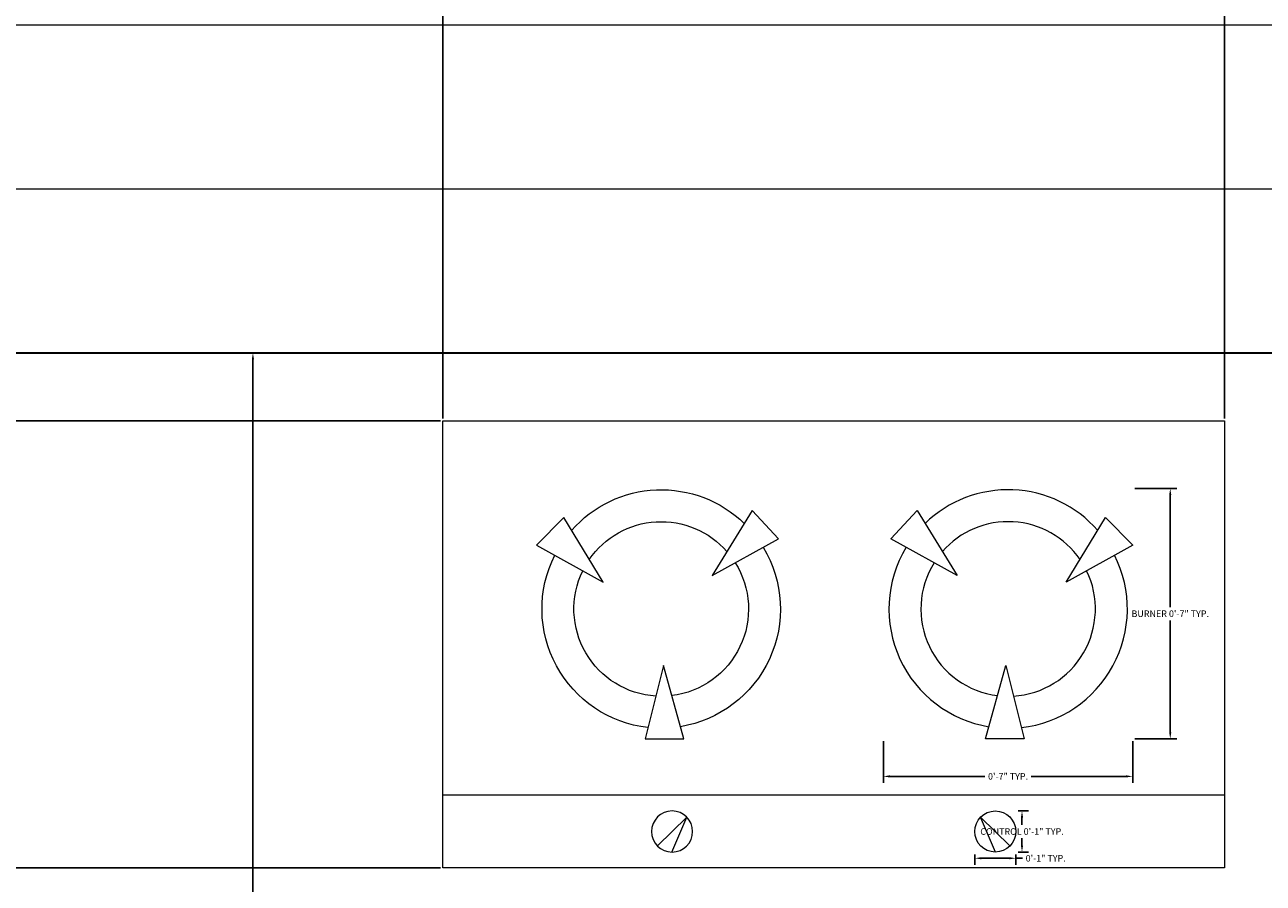
# Model space of a CAD drawing. Units: inches. Extents: x -5 to 482, y -460 to 66.
# Tile 26 of 31: x 72 to 106, y -10 to 13. Entities that reach past the tile are written whole.
import ezdxf

# ---------------------------------------------------------------- set-up
doc = ezdxf.new("R2010")
doc.units = ezdxf.units.IN
doc.header["$MEASUREMENT"] = 0
for name, color, linetype, lineweight in [('A-ANNO-DIMS', 2, 'Continuous', 18), ('A-EQPM', 8, 'Continuous', 18), ('A-GLAZ', 4, 'Continuous', 18), ('A-WALL', 7, 'Continuous', 35)]:
    doc.layers.add(name, color=color, linetype=linetype, lineweight=lineweight)
doc.styles.get("Standard").update_dxf_attribs({"font": 'arial.ttf'})
doc.dimstyles.get("Standard").update_dxf_attribs({"dimtxt": 0.18, "dimasz": 0.18, "dimexe": 0.18, "dimexo": 0.0625, "dimgap": 0.09, "dimtad": 0, "dimtih": 1, "dimtoh": 1, "dimdec": 0, "dimzin": 0, "dimdsep": 46, "dimlunit": 3, "dimtxsty": 'Standard', "dimcen": 0.09, "dimadec": 0, "dimazin": 0, "dimtfac": 1, "dimtdec": 0, "dimtofl": 0, "dimtmove": 0, "dimatfit": 3, "dimfxl": 1, "dimtolj": 1, "dimtzin": 0, "dimarcsym": 0})

# ---------------------------------------------------------------- blocks, each defined once
blk = doc.blocks.new('*D6')
at = {"layer": 'A-ANNO-DIMS', "color": 0, "lineweight": -2, "transparency": 16777216}
for p, q in [((78.657, 4.151), (78.326, 4.151)), ((78.506, 3.971), (78.506, -64.746)), ((78.506, -139.669), (78.506, -70.951)), ((78.657, -139.849), (78.326, -139.849))]:
    blk.add_line(p, q, dxfattribs=at)
at = {"layer": 'A-ANNO-DIMS', "color": 0, "transparency": 16777216}
for points in [[(78.476, 3.971), (78.536, 3.971), (78.506, 4.151)], [(78.476, -139.669), (78.536, -139.669), (78.506, -139.849)]]:
    blk.add_solid(points, dxfattribs=at)
at = {"layer": 'Defpoints', "color": 0, "transparency": 16777216}
for p in [(78.72, 4.151), (78.506, -139.849), (78.72, -139.849)]:
    blk.add_point(p, dxfattribs=at)
at = {"layer": 'A-ANNO-DIMS', "color": 0, "transparency": 16777216, "insert": (78.506, -67.849), "char_height": 6, "attachment_point": 5}
blk.add_mtext("\\A1;12'", dxfattribs=at)
blk = doc.blocks.new('WIN-GLAZ-60IN')
for p, q in [((0, 9), (60, 9)), ((0, 4.5), (60, 4.5)), ((60, 0), (0, 0))]:
    blk.add_line(p, q)
blk = doc.blocks.new('COOKTOP-BURNER')
for p, q in [((0.053, 5.484), (0.773, 6.261)), ((0.773, 6.261), (1.875, 4.484)), ((4.86, 4.295), (5.945, 6.068)), ((5.945, 6.068), (6.688, 5.312)), ((1.875, 4.484), (0.053, 5.484)), ((6.688, 5.312), (4.86, 4.295)), ((2.653, 0), (3.208, 2.016)), ((3.208, 2.016), (3.713, 0)), ((3.713, 0), (2.653, 0))]:
    blk.add_line(p, q)
for radius, start, end in [(3.271, 41.2225, 134.1627), (2.395, 34.5561, 138.8027), (3.271, 148.853, 260.7562), (2.395, 147.9778, 263.02), (3.271, 276.4005, 26.769), (2.395, 273.5753, 25.9207)]:
    blk.add_arc((3.27, 3.562), radius, start, end)
blk = doc.blocks.new('COOKTOP-CONTROL')
at = {"ltscale": 20}
for p, q in [((0.163, 0.962), (0.964, 0.167)), ((0.566, 0), (0.163, 0.962))]:
    blk.add_line(p, q, dxfattribs=at)
blk.add_circle((0.564, 0.564), 0.564, dxfattribs=at)
blk = doc.blocks.new('*D61')
at = {"layer": 'A-ANNO-DIMS', "color": 0, "lineweight": -2, "transparency": 16777216}
for p, q in [((102.71, 0.429), (103.858, 0.429)), ((103.678, 0.249), (103.678, -2.822)), ((103.678, -6.257), (103.678, -3.186)), ((102.71, -6.437), (103.858, -6.437))]:
    blk.add_line(p, q, dxfattribs=at)
at = {"layer": 'A-ANNO-DIMS', "color": 0, "transparency": 16777216}
for points in [[(103.648, 0.249), (103.708, 0.249), (103.678, 0.429)], [(103.648, -6.257), (103.708, -6.257), (103.678, -6.437)]]:
    blk.add_solid(points, dxfattribs=at)
at = {"layer": 'Defpoints', "color": 0, "transparency": 16777216}
for p in [(102.648, 0.429), (103.678, 0.429), (102.648, -6.437)]:
    blk.add_point(p, dxfattribs=at)
at = {"layer": 'A-ANNO-DIMS', "color": 0, "transparency": 16777216, "insert": (103.678, -3.004), "char_height": 0.18, "attachment_point": 5}
blk.add_mtext('\\A1;BURNER 0\'-7" TYP.', dxfattribs=at)
blk = doc.blocks.new('*D62')
at = {"layer": 'A-ANNO-DIMS', "color": 0, "lineweight": -2, "transparency": 16777216}
for p, q in [((95.806, -6.5), (95.806, -7.647)), ((102.648, -6.5), (102.648, -7.647)), ((95.986, -7.467), (98.588, -7.467)), ((102.468, -7.467), (99.865, -7.467))]:
    blk.add_line(p, q, dxfattribs=at)
at = {"layer": 'A-ANNO-DIMS', "color": 0, "transparency": 16777216}
for points in [[(95.986, -7.437), (95.986, -7.497), (95.806, -7.467)], [(102.468, -7.437), (102.468, -7.497), (102.648, -7.467)]]:
    blk.add_solid(points, dxfattribs=at)
at = {"layer": 'Defpoints', "color": 0, "transparency": 16777216}
for p in [(95.806, -6.437), (102.648, -6.437), (102.648, -7.467)]:
    blk.add_point(p, dxfattribs=at)
at = {"layer": 'A-ANNO-DIMS', "color": 0, "transparency": 16777216, "insert": (99.227, -7.467), "char_height": 0.18, "attachment_point": 5}
blk.add_mtext('\\A1;0\'-7" TYP.', dxfattribs=at)
blk = doc.blocks.new('*D63')
at = {"layer": 'A-ANNO-DIMS', "color": 0, "lineweight": -2, "transparency": 16777216}
for p, q in [((99.503, -8.415), (99.79, -8.415)), ((99.61, -8.595), (99.61, -8.796)), ((99.61, -9.363), (99.61, -9.162)), ((99.503, -9.543), (99.79, -9.543))]:
    blk.add_line(p, q, dxfattribs=at)
at = {"layer": 'A-ANNO-DIMS', "color": 0, "transparency": 16777216}
for points in [[(99.58, -8.595), (99.64, -8.595), (99.61, -8.415)], [(99.58, -9.363), (99.64, -9.363), (99.61, -9.543)]]:
    blk.add_solid(points, dxfattribs=at)
at = {"layer": 'Defpoints', "color": 0, "transparency": 16777216}
for p in [(99.441, -8.415), (99.61, -8.415), (99.441, -9.543)]:
    blk.add_point(p, dxfattribs=at)
at = {"layer": 'A-ANNO-DIMS', "color": 0, "transparency": 16777216, "insert": (99.61, -8.979), "char_height": 0.18, "attachment_point": 5}
blk.add_mtext('\\A1;CONTROL 0\'-1" TYP.', dxfattribs=at)
blk = doc.blocks.new('*D64')
at = {"layer": 'A-ANNO-DIMS', "color": 0, "lineweight": -2, "transparency": 16777216}
for p, q in [((98.313, -9.606), (98.313, -9.892)), ((98.493, -9.712), (99.261, -9.712)), ((99.441, -9.606), (99.441, -9.892)), ((99.441, -9.712), (99.621, -9.712))]:
    blk.add_line(p, q, dxfattribs=at)
at = {"layer": 'A-ANNO-DIMS', "color": 0, "transparency": 16777216}
for points in [[(98.493, -9.682), (98.493, -9.742), (98.313, -9.712)], [(99.261, -9.682), (99.261, -9.742), (99.441, -9.712)]]:
    blk.add_solid(points, dxfattribs=at)
at = {"layer": 'Defpoints', "color": 0, "transparency": 16777216}
for p in [(98.313, -9.543), (99.441, -9.543), (99.441, -9.712)]:
    blk.add_point(p, dxfattribs=at)
at = {"layer": 'A-ANNO-DIMS', "color": 0, "transparency": 16777216, "insert": (100.26, -9.712), "char_height": 0.18, "attachment_point": 5}
blk.add_mtext('\\A1;0\'-1" TYP.', dxfattribs=at)
blk = doc.blocks.new('*D69')
at = {"layer": 'A-ANNO-DIMS', "color": 0, "lineweight": -2, "transparency": 16777216}
for p, q in [((83.715, 2.351), (83.715, 50.931)), ((83.895, 50.751), (93.912, 50.751)), ((104.991, 50.751), (94.973, 50.751)), ((105.171, 2.351), (105.171, 50.931))]:
    blk.add_line(p, q, dxfattribs=at)
at = {"layer": 'A-ANNO-DIMS', "color": 0, "transparency": 16777216}
for points in [[(83.895, 50.781), (83.895, 50.721), (83.715, 50.751)], [(104.991, 50.781), (104.991, 50.721), (105.171, 50.751)]]:
    blk.add_solid(points, dxfattribs=at)
at = {"layer": 'Defpoints', "color": 0, "transparency": 16777216}
for p in [(105.171, 50.751), (83.715, 2.288), (105.171, 2.288)]:
    blk.add_point(p, dxfattribs=at)
at = {"layer": 'A-ANNO-DIMS', "color": 0, "transparency": 16777216, "insert": (94.443, 50.751), "char_height": 0.18, "attachment_point": 5}
blk.add_mtext('\\A1;1\'-9 1/2"', dxfattribs=at)
blk = doc.blocks.new('*D70')
at = {"layer": 'A-ANNO-DIMS', "color": 0, "lineweight": -2, "transparency": 16777216}
for p, q in [((83.652, 2.288), (-4.903, 2.288)), ((-4.723, 2.108), (-4.723, -3.659)), ((-4.723, -9.792), (-4.723, -4.025)), ((83.652, -9.972), (-4.903, -9.972))]:
    blk.add_line(p, q, dxfattribs=at)
at = {"layer": 'A-ANNO-DIMS', "color": 0, "transparency": 16777216}
for points in [[(-4.753, 2.108), (-4.693, 2.108), (-4.723, 2.288)], [(-4.753, -9.792), (-4.693, -9.792), (-4.723, -9.972)]]:
    blk.add_solid(points, dxfattribs=at)
at = {"layer": 'Defpoints', "color": 0, "transparency": 16777216}
for p in [(83.715, 2.288), (-4.723, -9.972), (83.715, -9.972)]:
    blk.add_point(p, dxfattribs=at)
at = {"layer": 'A-ANNO-DIMS', "color": 0, "transparency": 16777216, "insert": (-4.723, -3.842), "char_height": 0.18, "attachment_point": 5}
blk.add_mtext('\\A1;1\'-0 1/2"', dxfattribs=at)

msp = doc.modelspace()

# ---------------------------------------------------------------- linework, layer by layer
at = {"layer": 'A-EQPM'}
msp.add_line((105.171, -7.98), (83.715, -7.98), dxfattribs=at)
msp.add_lwpolyline([(83.715, 2.288), (105.171, 2.288), (105.171, -9.972), (83.715, -9.972)], close=True, dxfattribs=at)
at = {"layer": 'A-WALL'}
msp.add_line((41.877, 4.151), (149.877, 4.151), dxfattribs=at)

# ---------------------------------------------------------------- block references
at = {"layer": 'A-EQPM', "extrusion": (0, 0, -1), "zscale": -1}
for name, p in [('COOKTOP-BURNER', (-92.98, -6.437)), ('COOKTOP-CONTROL', (-90.572, -9.543))]:
    msp.add_blockref(name, p, dxfattribs=at)
at = {"layer": 'A-EQPM'}
for name, p in [('COOKTOP-BURNER', (95.96, -6.437)), ('COOKTOP-CONTROL', (98.313, -9.543))]:
    msp.add_blockref(name, p, dxfattribs=at)
at = {"layer": 'A-GLAZ'}
msp.add_blockref('WIN-GLAZ-60IN', (65.877, 4.151), dxfattribs=at)

# ---------------------------------------------------------------- dimensions: what is measured, and where the dimension line sits
at = {"layer": 'A-ANNO-DIMS'}
dim = msp.add_linear_dim(base=(105.171, 50.751), p1=(83.715, 2.288), p2=(105.171, 2.288), dimstyle='Standard', override={"dimdec": 1, "dimlfac": 1, "dimrnd": 0, "dimzin": 1, "dimdsep": 46, "dimlunit": 4, "dimfrac": 2}, dxfattribs=at)
dim.commit()
dim.dimension.update_dxf_attribs({"geometry": '*D69', "text_midpoint": (94.443, 50.751)})
for base, p1, p2, override, picture, middle in [((78.506, -139.849), (78.72, 4.151), (78.72, -139.849), {"dimtxt": 6, "dimclrd": 0, "dimclre": 0, "dimclrt": 0}, '*D6', (78.506, -67.849)), ((-4.723, -9.972), (83.715, 2.288), (83.715, -9.972), {"dimdec": 1, "dimlfac": 1, "dimrnd": 0, "dimzin": 1, "dimdsep": 46, "dimlunit": 4, "dimfrac": 2}, '*D70', (-4.723, -3.842))]:
    dim = msp.add_linear_dim(base=base, p1=p1, p2=p2, angle=90, dimstyle='Standard', override=override, dxfattribs=at)
    dim.commit()
    dim.dimension.update_dxf_attribs({"geometry": picture, "text_midpoint": middle})
for base, p1, p2, text, picture, middle in [((103.678, 0.429), (102.648, -6.437), (102.648, 0.429), 'BURNER <> TYP.', '*D61', (103.678, -3.004)), ((99.61, -8.415), (99.441, -9.543), (99.441, -8.415), 'CONTROL <> TYP.', '*D63', (99.61, -8.979))]:
    dim = msp.add_linear_dim(base=base, p1=p1, p2=p2, angle=90, text=text, dimstyle='Standard', override={"dimdec": 1, "dimlfac": 1, "dimrnd": 0, "dimzin": 1, "dimdsep": 46, "dimlunit": 4, "dimfrac": 2}, dxfattribs=at)
    dim.commit()
    dim.dimension.update_dxf_attribs({"geometry": picture, "text_midpoint": middle})
for base, p1, p2, picture, middle in [((102.648, -7.467), (95.806, -6.437), (102.648, -6.437), '*D62', (99.227, -7.467)), ((99.441, -9.712), (98.313, -9.543), (99.441, -9.543), '*D64', (100.26, -9.712))]:
    dim = msp.add_linear_dim(base=base, p1=p1, p2=p2, text='<> TYP.', dimstyle='Standard', override={"dimdec": 1, "dimlfac": 1, "dimrnd": 0, "dimzin": 1, "dimdsep": 46, "dimlunit": 4, "dimfrac": 2}, dxfattribs=at)
    dim.commit()
    dim.dimension.update_dxf_attribs({"geometry": picture, "text_midpoint": middle})

doc.saveas('drawing.dxf')
